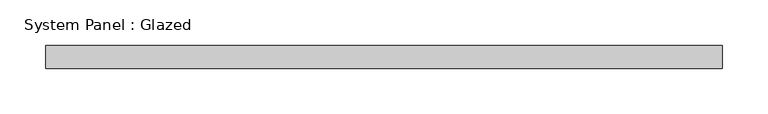
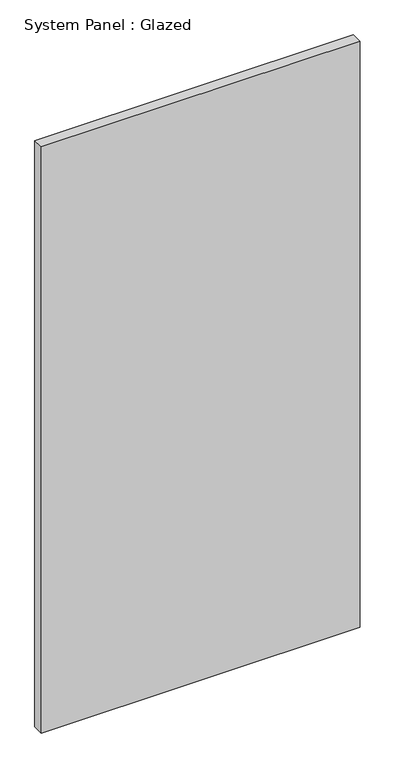
"""IFC4 building model written with IfcOpenShell, lengths in millimetres: plate geometry, System Panel : Glazed."""

from ifc_helpers import new_model, si_unit, origin, origin_with_axes, place, context, project, spatial, polyline, outline, extrude, source, transform, mapped, element, save


def system_panel_glazed_d02f90d0(model_context):
    return source(origin(), model_context, "Body", "SweptSolid", [
        extrude(outline(polyline([(371.475, 19.05), (-371.475, 19.05), (-371.475, 44.45), (371.475, 44.45), (371.475, 19.05)])), origin_with_axes(), (0.0, 0.0, 1.0), 1444.0246189),
    ])


if __name__ == "__main__":
    model = new_model("IFC4")
    model_context = context("Model", 3, world=origin())
    ifc_project = project(units=[si_unit("LENGTHUNIT", "METRE", prefix="MILLI")], contexts=[model_context])
    site = spatial("IfcSite", under=ifc_project)
    building = spatial("IfcBuilding", under=site)
    placement = place(None, origin())
    system_panel_glazed_shape = system_panel_glazed_d02f90d0(model_context)
    element("IfcPlate", 1, ObjectType="System Panel : Glazed", at=placement, inside=building, context=model_context, shape_type="MappedRepresentation", body=[
        mapped(system_panel_glazed_shape, transform((0.0, 0.0, 0.0), x_axis=(1.0, 0.0, 0.0), y_axis=(0.0, 1.0, 0.0), z_axis=(0.0, 0.0, 1.0))),
    ])
    save(model, "model.ifc")

# Revit data of these elements
# Type "System Panel : Glazed"
#   Construction Type Id = "GSP4R"
#   Analytic Construction = "1/8 in Pilkington single glazing"
#   Visual Light Transmittance = 0.9
#   Solar Heat Gain Coefficient = 0.86
#   Heat Transfer Coefficient (U) = 1.18115 BTU/(h·ft²·°F)
#   Define Thermal Properties by = 1
# Element 1 (IfcPlate, "System Panel : Glazed")
#   Materials on its faces: "Glass"
# Materials
#   "Glass": class "Glass", colour RGB 0 128 192, transparency 0.75, Description = "Soda Lime Glass", Cost = 0
